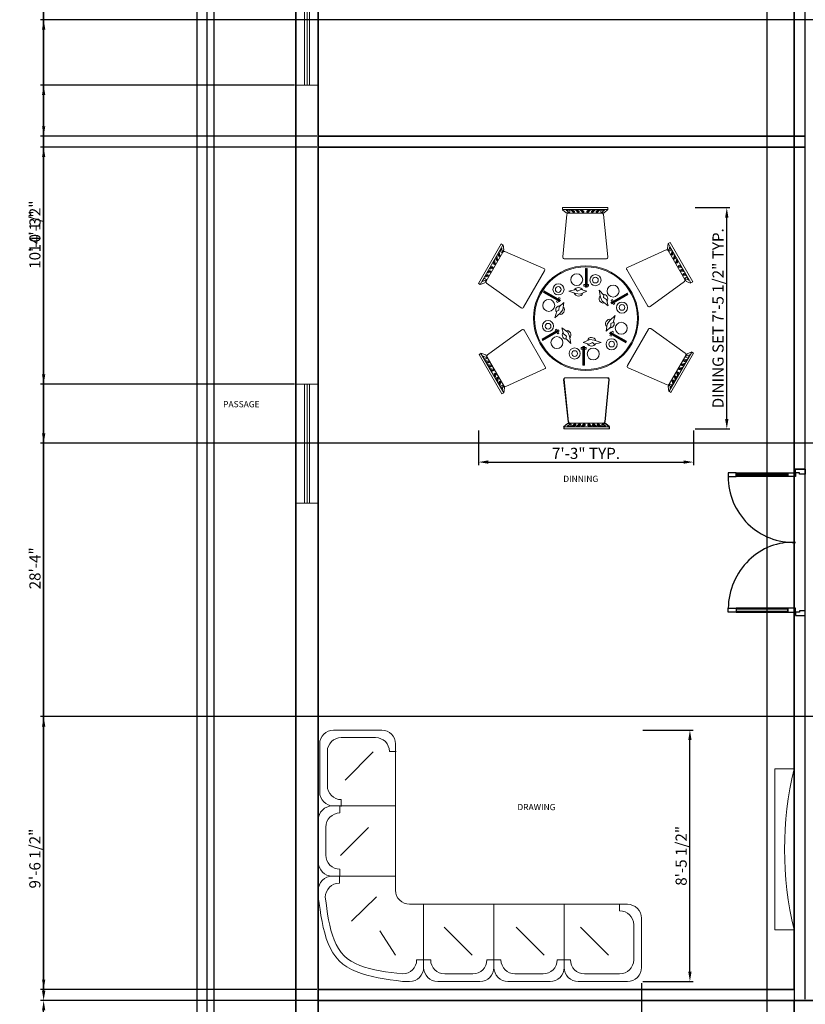
# Model space of a CAD drawing. Units: inches. Extents: x 1239 to 2276906, y 2273 to 321338.
# Tile 10 of 23: x 1239 to 1556, y 2629 to 3026. Entities that reach past the tile are written whole.
import ezdxf

# ---------------------------------------------------------------- set-up
doc = ezdxf.new("R2010")
doc.units = ezdxf.units.IN
for name, color, linetype, lineweight in [('A-ANNO-DIMS', 2, 'Continuous', 18), ('A-AREA-IDEN', 7, 'Continuous', 18), ('A-FLOR-CASE', 8, 'Continuous', 18), ('A-FLOR-PORCH', 7, 'Continuous', 25), ('A-FURN', 8, 'Continuous', 13), ('C-PROP', 7, 'Continuous', 25), ('DOOR', 1, 'Continuous', 25), ('wall', 7, 'Continuous', 35), ('WINDOW', 50, 'Continuous', 18)]:
    doc.layers.add(name, color=color, linetype=linetype, lineweight=lineweight)
doc.styles.get("Standard").update_dxf_attribs({"font": 'arial.ttf'})
doc.dimstyles.new('ISO-25', dxfattribs={"dimtxt": 4.5, "dimasz": 4, "dimexe": 1.25, "dimexo": 0.625, "dimtad": 1, "dimdec": 1, "dimlunit": 3, "dimtxsty": 'Standard', "dimcen": 2.5, "dimadec": 0, "dimazin": 0, "dimtfac": 1, "dimtdec": 1, "dimtmove": 0, "dimatfit": 3, "dimfxl": 1, "dimarcsym": 0})

# ---------------------------------------------------------------- blocks, each defined once
blk = doc.blocks.new('A$C4B324E0D')
for points in [[(-0.4032, -0.0374), (-0.3959, 0.0153), (-0.3883, 0.0678), (-0.3801, 0.1195), (-0.3709, 0.1704), (-0.3605, 0.22), (-0.3485, 0.2679), (-0.3346, 0.314), (-0.3185, 0.3579), (-0.2998, 0.3993), (-0.2783, 0.4378), (-0.2537, 0.4731), (-0.2255, 0.5049), (-0.1936, 0.5331), (-0.1583, 0.5578), (-0.1198, 0.5793), (-0.0785, 0.5979), (-0.0346, 0.614), (0.0115, 0.628), (0.0595, 0.64), (0.1091, 0.6504), (0.1599, 0.6595), (0.2117, 0.6678), (0.2641, 0.6753), (0.3168, 0.6826)], [(0.3768, 0.6826), (0.3168, 0.6826)], [(0.9768, 0.6826), (0.6168, 0.6826)], [(1.5769, 0.6826), (1.2168, 0.6826)], [(1.8168, 0.6826), (2.2368, 0.6826)], [(-0.3432, -0.0374), (-0.3369, 0.0114), (-0.3303, 0.0599), (-0.3232, 0.1078), (-0.3151, 0.1548), (-0.3059, 0.2006), (-0.2951, 0.2449), (-0.2826, 0.2874), (-0.2681, 0.3278), (-0.2511, 0.3658), (-0.2315, 0.4011), (-0.2089, 0.4335), (-0.1831, 0.4625), (-0.1538, 0.488), (-0.1214, 0.5102), (-0.086, 0.5294), (-0.0479, 0.546), (-0.0075, 0.5602), (0.035, 0.5722), (0.0793, 0.5825), (0.125, 0.5914), (0.172, 0.599), (0.2198, 0.6057), (0.2682, 0.6119), (0.3168, 0.6177)], [(0.3168, 0.6177), (0.3168, 0.6177)], [(0.9168, 0.6177), (0.6768, 0.6177)], [(1.5168, 0.6177), (1.2768, 0.6177)], [(2.1704, 0.6177), (1.8704, 0.6177)], [(0.4968, 0.0226), (0.4968, 0.5626)], [(0.4968, 0.5626), (0.4968, 0.0226), (1.0968, 0.0226)], [(1.0968, 0.5626), (1.0968, 0.0226), (1.6968, 0.0226)], [(1.0968, 0.0226), (1.0968, 0.5626)], [(1.6968, 0.0226), (1.6968, 0.5626)], [(2.2368, 0.0226), (1.6968, 0.0226), (1.6968, 0.5626)], [(2.3569, 0.5626), (2.3569, 0.1426)], [(0.255, 0.4573), (0.1211, 0.2495)], [(0.4968, 0.4977), (0.4368, 0.4977), (0.4368, 0.4977)], [(0.5569, 0.4977), (0.5569, 0.4977), (0.4968, 0.4977)], [(0.9111, 0.4573), (0.6711, 0.2173)], [(1.0968, 0.4977), (1.0368, 0.4977), (1.0368, 0.4977)], [(1.1569, 0.4977), (1.1569, 0.4977), (1.0968, 0.4977)], [(1.527, 0.4573), (1.287, 0.2173)], [(1.6969, 0.4977), (1.6368, 0.4977), (1.6368, 0.4977)], [(1.7504, 0.4977), (1.7504, 0.4977), (1.6904, 0.4977)], [(2.0759, 0.4573), (1.8359, 0.2173)], [(2.2904, 0.1977), (2.2904, 0.4977)], [(-0.1199, 0.1664), (0.0943, -0.0414)], [(0.4968, 0.0226), (0.3768, 0.0226)], [(2.1704, 0.0177), (2.1704, 0.0777), (2.1704, 0.0777)], [(-0.4032, -0.0974), (-0.4032, -0.0374)], [(-0.3432, -0.0374), (-0.3432, -0.0374)], [(-0.2232, -0.2174), (-0.2232, -0.1574), (-0.2232, -0.1574)], [(0.2568, -0.0974), (0.2568, -0.2174)], [(-0.2832, -0.8174), (0.2568, -0.8174), (0.2568, -0.2174)], [(0.2568, -0.2174), (-0.2832, -0.2174)], [(0.2568, -0.2174), (-0.2832, -0.2174)], [(-0.2183, -0.2174), (-0.2183, -0.2774), (-0.2183, -0.2774)], [(-0.4032, -0.3374), (-0.4032, -0.6974)], [(-0.3383, -0.3974), (-0.3383, -0.6374)], [(-0.2136, -0.3946), (0.0264, -0.6346)], [(0.2568, -0.8174), (-0.2832, -0.8174)], [(-0.2732, -0.8174), (0.2568, -0.8174), (0.2568, -1.3475)], [(-0.2183, -0.7574), (-0.2183, -0.7574), (-0.2183, -0.8174)], [(-0.208, -0.8126), (-0.208, -0.8715), (-0.208, -0.8715)], [(0.2568, -0.8174), (0.2568, -1.3475)], [(-0.391, -1.3475), (-0.391, -0.9352)], [(-0.3258, -0.9893), (-0.3258, -1.2838)], [(-0.1734, -1.0387), (0.0666, -1.2787)], [(0.2043, -1.2838), (0.2043, -1.2838), (0.2632, -1.2838)], [(-0.208, -1.4016), (0.0865, -1.4016)], [(0.1391, -1.4653), (-0.2732, -1.4653)]]:
    blk.add_lwpolyline(points)
for centre, radius, start, end in [((0.3768, 0.5626), 0.12, 0, 90), ((0.6168, 0.5626), 0.12, 90, 180), ((0.9768, 0.5626), 0.12, 0, 90), ((1.2168, 0.5626), 0.12, 90, 180), ((1.5769, 0.5626), 0.12, 0, 90), ((1.8168, 0.5626), 0.12, 90, 180), ((2.2368, 0.5626), 0.12, 0, 90), ((0.3168, 0.4977), 0.12, 0, 90), ((0.6768, 0.4977), 0.12, 90, 180), ((0.9168, 0.4977), 0.12, 0, 90), ((1.2768, 0.4977), 0.12, 90, 180), ((1.5168, 0.4977), 0.12, 0, 90), ((1.8704, 0.4977), 0.12, 90, 180), ((2.1704, 0.4977), 0.12, 0, 90), ((2.1704, 0.1977), 0.12, 270, 0), ((2.2368, 0.1426), 0.12, 270, 0), ((0.3768, -0.0974), 0.12, 90, 180), ((-0.2232, -0.0374), 0.12, 180, 270), ((-0.2832, -0.0974), 0.12, 179.9997, 270), ((-0.2832, -0.3374), 0.12, 90, 180), ((-0.2183, -0.3974), 0.12, 90, 180), ((-0.2183, -0.6374), 0.12, 180, 270), ((-0.2832, -0.6974), 0.12, 179.9997, 270), ((-0.2732, -0.9352), 0.1178, 90, 180), ((-0.208, -0.9893), 0.1178, 90, 180), ((-0.208, -1.2838), 0.1178, 180, 270), ((0.0865, -1.2838), 0.1178, 270, 0), ((-0.2732, -1.3475), 0.1178, 179.9997, 270), ((0.1391, -1.3475), 0.1178, 270, 0)]:
    blk.add_arc(centre, radius, start, end)
blk = doc.blocks.new('A$C58C6152E')
at = {"xscale": 1.5, "yscale": 1.5, "zscale": 1.5, "rotation": 90}
blk.add_blockref('A$C4B324E0D', (1.024, 0.605), dxfattribs=at)
blk = doc.blocks.new('A$C15DC316E')
at = {"xscale": -1, "rotation": 270}
blk.add_blockref('A$C58C6152E', (0, 0), dxfattribs=at)
blk = doc.blocks.new('A$C45501D90')
for p, q in [((-242, 1134), (224, 1134)), ((-242, 1113), (-242, 1134)), ((224, 1113), (-242, 1113)), ((-242, 1111), (-202, 1079)), ((224, 1113), (187, 1079)), ((224, 1134), (224, 1113)), ((-197, 1062), (-239, 628)), ((-204, 1106), (-166, 1108)), ((-169, 1081), (-204, 1106)), ((-202, 1079), (-169, 1081)), ((162, 1076), (-181, 1076)), ((-166, 1108), (-167, 1086)), ((-156, 1110), (-132, 1086)), ((-119, 1086), (-143, 1108)), ((-143, 1108), (-134, 1108)), ((-134, 1108), (-122, 1098)), ((-132, 1086), (-119, 1086)), ((-122, 1098), (-119, 1102)), ((-119, 1102), (-118, 1087)), ((-108, 1110), (-84, 1086)), ((-71, 1086), (-95, 1108)), ((-95, 1108), (-86, 1108)), ((-86, 1108), (-75, 1098)), ((-84, 1086), (-71, 1086)), ((-75, 1098), (-71, 1102)), ((-71, 1102), (-70, 1087)), ((-60, 1110), (-36, 1086)), ((-23, 1086), (-47, 1108)), ((-47, 1108), (-38, 1108)), ((-38, 1108), (-27, 1098)), ((-36, 1086), (-23, 1086)), ((-27, 1098), (-23, 1102)), ((-23, 1102), (-22, 1087)), ((8, 1102), (7, 1087)), ((8, 1086), (32, 1108)), ((12, 1098), (8, 1102)), ((21, 1086), (8, 1086)), ((23, 1108), (12, 1098)), ((45, 1110), (21, 1086)), ((32, 1108), (23, 1108)), ((56, 1102), (55, 1087)), ((56, 1086), (80, 1108)), ((60, 1098), (56, 1102)), ((69, 1086), (56, 1086)), ((71, 1108), (60, 1098)), ((93, 1110), (69, 1086)), ((80, 1108), (71, 1108)), ((104, 1102), (103, 1087)), ((104, 1086), (128, 1108)), ((107, 1098), (104, 1102)), ((117, 1086), (104, 1086)), ((119, 1108), (107, 1098)), ((141, 1110), (117, 1086)), ((128, 1108), (119, 1108)), ((189, 1106), (151, 1108)), ((151, 1108), (152, 1086)), ((154, 1081), (189, 1106)), ((187, 1079), (154, 1081)), ((225, 628), (178, 1062)), ((-1103, 357), (-870, 761)), ((-852, 750), (-1085, 347)), ((-864, 717), (-884, 684)), ((-870, 761), (-852, 750)), ((-859, 674), (-864, 717)), ((-849, 752), (-841, 702)), ((841, 765), (834, 715)), ((834, 715), (852, 687)), ((843, 766), (861, 776)), ((1076, 362), (843, 766)), ((852, 687), (856, 730)), ((856, 730), (877, 697)), ((861, 776), (1094, 373)), ((-851, 678), (-1023, 381)), ((-919, 624), (-924, 615)), ((-924, 615), (-921, 601)), ((-912, 592), (-919, 624)), ((-914, 635), (-906, 603)), ((-898, 642), (-902, 641)), ((-902, 641), (-890, 633)), ((-895, 665), (-900, 657)), ((-900, 657), (-898, 642)), ((-888, 633), (-895, 665)), ((-890, 677), (-882, 644)), ((-882, 644), (-888, 633)), ((-884, 684), (-864, 675)), ((-841, 702), (-859, 674)), ((-431, 509), (-831, 685)), ((-223, 610), (209, 610)), ((821, 702), (424, 521)), ((1013, 398), (841, 695)), ((877, 697), (857, 688)), ((883, 690), (874, 657)), ((874, 657), (881, 646)), ((881, 646), (888, 678)), ((894, 654), (883, 646)), ((888, 678), (893, 670)), ((893, 670), (890, 655)), ((890, 655), (894, 654)), ((907, 648), (898, 616)), ((898, 616), (904, 605)), ((904, 605), (912, 637)), ((918, 613), (907, 604)), ((912, 637), (917, 628)), ((917, 628), (914, 614)), ((914, 614), (918, 613)), ((931, 607), (922, 574)), ((-991, 503), (-958, 511)), ((-952, 522), (-983, 513)), ((-983, 513), (-978, 521)), ((-978, 521), (-965, 526)), ((-965, 526), (-966, 530)), ((-966, 530), (-953, 525)), ((-958, 511), (-952, 522)), ((-945, 559), (-950, 558)), ((-950, 558), (-938, 550)), ((-943, 582), (-948, 574)), ((-948, 574), (-945, 559)), ((-936, 550), (-943, 582)), ((-938, 594), (-930, 561)), ((-930, 561), (-936, 550)), ((-921, 601), (-926, 600)), ((-926, 600), (-914, 591)), ((-906, 603), (-912, 592)), ((-6, 509, 91), (0, 509, 91)), ((-6, 318, 91), (-6, 509, 91)), ((0, 509, 91), (0, 318, 91)), ((6, 318, 91), (6, 509, 91)), ((6, 509, 91), (12, 509, 91)), ((12, 509, 91), (12, 318, 91)), ((922, 574), (928, 563)), ((928, 563), (936, 595)), ((942, 571), (931, 563)), ((936, 595), (941, 587)), ((941, 587), (938, 572)), ((938, 572), (942, 571)), ((951, 524), (944, 535)), ((944, 535), (976, 526)), ((958, 543), (945, 538)), ((983, 516), (951, 524)), ((957, 539), (958, 543)), ((971, 534), (957, 539)), ((976, 526), (971, 534)), ((-1060, 377), (-1042, 411)), ((-1042, 411), (-1024, 398)), ((-1039, 420), (-1006, 428)), ((-1000, 440), (-1031, 430)), ((-1031, 430), (-1026, 438)), ((-1026, 438), (-1012, 443)), ((-1015, 461), (-982, 470)), ((-1012, 443), (-1014, 448)), ((-1014, 448), (-1000, 442)), ((-976, 481), (-1007, 471)), ((-1007, 471), (-1002, 480)), ((-1006, 428), (-1000, 440)), ((-1002, 480), (-989, 485)), ((-989, 485), (-990, 489)), ((-990, 489), (-976, 483)), ((-982, 470), (-976, 481)), ((-640, 112), (-424, 486)), ((417, 498), (633, 124)), ((968, 494), (1000, 484)), ((975, 483), (968, 494)), ((982, 502), (969, 496)), ((1007, 474), (975, 483)), ((981, 498), (982, 502)), ((995, 493), (981, 498)), ((999, 441), (992, 453)), ((992, 453), (1024, 443)), ((1006, 461), (993, 455)), ((1000, 484), (995, 493)), ((1031, 433), (999, 441)), ((1005, 456), (1006, 461)), ((1019, 451), (1005, 456)), ((1028, 377), (1013, 407)), ((1013, 407), (1053, 390)), ((1035, 424), (1016, 411)), ((1024, 443), (1019, 451)), ((1053, 390), (1035, 424)), ((-1085, 347), (-1103, 357)), ((-1083, 346), (-1036, 364)), ((-1020, 394), (-1060, 377)), ((-1036, 364), (-1020, 394)), ((-1018, 360), (-663, 107)), ((-22, 329, 91), (-22, 345, 91)), ((-22, 345, 91), (-6, 345, 91)), ((-6, 329, 91), (-22, 329, 91)), ((0, 318, 91), (-6, 318, 91)), ((0, 345, 91), (6, 345, 91)), ((6, 329, 91), (0, 329, 91)), ((12, 318, 91), (6, 318, 91)), ((12, 345, 91), (27, 345, 91)), ((27, 329, 91), (12, 329, 91)), ((27, 345, 91), (27, 329, 91)), ((656, 119), (1008, 377)), ((1076, 359), (1028, 377)), ((1094, 373), (1076, 362)), ((-436, 265, 91), (-433, 271, 91)), ((-271, 170, 91), (-436, 265, 91)), ((-433, 271, 91), (-268, 175, 91)), ((-431, 275, 91), (-428, 280, 91)), ((-265, 180, 91), (-431, 275, 91)), ((-428, 280, 91), (-262, 185, 91)), ((-286, 198, 91), (-278, 212, 91)), ((-278, 212, 91), (-264, 204, 91)), ((-264, 204, 91), (-272, 191, 91)), ((-175, 276, 91), (-105, 293, 91)), ((-103, 252, 91), (-175, 276, 91)), ((-105, 293, 91), (-86, 278, 91)), ((-60, 246, 91), (-103, 252, 91)), ((-86, 278, 91), (-52, 294, 91)), ((9, 276, 91), (-60, 246, 91)), ((-52, 294, 91), (9, 276, 91)), ((134, 288, 91), (184, 236, 91)), ((150, 214, 91), (134, 288, 91)), ((166, 173, 91), (150, 214, 91)), ((184, 236, 91), (181, 211, 91)), ((181, 211, 91), (211, 190, 91)), ((255, 162, 91), (421, 257, 91)), ((424, 252, 91), (258, 157, 91)), ((261, 152, 91), (426, 248, 91)), ((429, 242, 91), (264, 147, 91)), ((421, 257, 91), (424, 252, 91)), ((426, 248, 91), (429, 242, 91)), ((-303, 169, 91), (-294, 183, 91)), ((-289, 161, 91), (-303, 169, 91)), ((-291, 188, 91), (-289, 193, 91)), ((-281, 176, 91), (-289, 161, 91)), ((-275, 185, 91), (-278, 181, 91)), ((-277, 81, 91), (-274, 118, 91)), ((-274, 118, 91), (-227, 162, 91)), ((-268, 175, 91), (-271, 170, 91)), ((-262, 185, 91), (-265, 180, 91)), ((-227, 162, 91), (-236, 87, 91)), ((227, 128, 91), (166, 173, 91)), ((211, 190, 91), (227, 128, 91)), ((258, 157, 91), (255, 162, 91)), ((257, 182, 91), (270, 190, 91)), ((265, 168, 91), (257, 182, 91)), ((264, 147, 91), (261, 152, 91)), ((271, 158, 91), (268, 162, 91)), ((270, 190, 91), (278, 175, 91)), ((281, 139, 91), (274, 153, 91)), ((281, 170, 91), (284, 165, 91)), ((295, 147, 91), (281, 139, 91)), ((287, 160, 91), (295, 147, 91)), ((-320, 2, 91), (-299, 72, 91)), ((-263, 53, 91), (-320, 2, 91)), ((-299, 72, 91), (-277, 81, 91)), ((-236, 87, 91), (-263, 53, 91)), ((243, -25, 91), (299, 26, 91)), ((299, 26, 91), (279, -44, 91)), ((-247, -100, 91), (-187, -145, 91)), ((-232, -162, 91), (-247, -100, 91)), ((207, -134, 91), (216, -60, 91)), ((253, -90, 91), (207, -134, 91)), ((216, -60, 91), (243, -25, 91)), ((256, -53, 91), (253, -90, 91)), ((279, -44, 91), (256, -53, 91)), ((-656, -119), (-1008, -377)), ((-417, -498), (-633, -124)), ((-450, -214, 91), (-284, -119, 91)), ((-281, -124, 91), (-447, -220, 91)), ((-444, -224, 91), (-279, -129, 91)), ((-276, -134, 91), (-441, -229, 91)), ((-315, -119, 91), (-302, -111, 91)), ((-307, -132, 91), (-315, -119, 91)), ((-302, -142, 91), (-304, -137, 91)), ((-302, -111, 91), (-294, -125, 91)), ((-290, -162, 91), (-299, -147, 91)), ((-291, -130, 91), (-288, -134, 91)), ((-277, -154, 91), (-290, -162, 91)), ((-285, -140, 91), (-277, -154, 91)), ((-284, -119, 91), (-281, -124, 91)), ((-279, -129, 91), (-276, -134, 91)), ((-201, -183, 91), (-232, -162, 91)), ((-205, -208, 91), (-201, -183, 91)), ((-187, -145, 91), (-170, -186, 91)), ((-170, -186, 91), (-155, -260, 91)), ((242, -157, 91), (245, -152, 91)), ((407, -252, 91), (242, -157, 91)), ((244, -176, 91), (252, -163, 91)), ((257, -184, 91), (244, -176, 91)), ((245, -152, 91), (410, -247, 91)), ((248, -147, 91), (251, -142, 91)), ((413, -243, 91), (248, -147, 91)), ((251, -142, 91), (416, -237, 91)), ((255, -157, 91), (257, -153, 91)), ((265, -170, 91), (257, -184, 91)), ((260, -148, 91), (269, -133, 91)), ((271, -160, 91), (268, -165, 91)), ((269, -133, 91), (282, -141, 91)), ((282, -141, 91), (274, -155, 91)), ((640, -112), (424, -486)), ((1018, -360), (663, -107)), ((-447, -220, 91), (-450, -214, 91)), ((-441, -229, 91), (-444, -224, 91)), ((-155, -260, 91), (-205, -208, 91)), ((-48, -317, 91), (-48, -301, 91)), ((-48, -301, 91), (-32, -301, 91)), ((-32, -481, 91), (-32, -290, 91)), ((-32, -290, 91), (-26, -290, 91)), ((-30, -248, 91), (39, -218, 91)), ((32, -266, 91), (-30, -248, 91)), ((-26, -290, 91), (-26, -481, 91)), ((-26, -301, 91), (-21, -301, 91)), ((-21, -481, 91), (-21, -290, 91)), ((-21, -290, 91), (-15, -290, 91)), ((-15, -290, 91), (-15, -481, 91)), ((-15, -301, 91), (2, -301, 91)), ((2, -301, 91), (2, -317, 91)), ((65, -250, 91), (32, -266, 91)), ((39, -218, 91), (83, -224, 91)), ((84, -265, 91), (65, -250, 91)), ((83, -224, 91), (155, -248, 91)), ((155, -248, 91), (84, -265, 91)), ((410, -247, 91), (407, -252, 91)), ((416, -237, 91), (413, -243, 91)), ((-1094, -373), (-1076, -362)), ((-861, -776), (-1094, -373)), ((-1076, -359), (-1028, -377)), ((-1076, -362), (-843, -766)), ((-1053, -390), (-1035, -424)), ((-1013, -407), (-1053, -390)), ((-1028, -377), (-1013, -407)), ((-1013, -398), (-841, -695)), ((-32, -317, 91), (-48, -317, 91)), ((-21, -317, 91), (-26, -317, 91)), ((2, -317, 91), (-15, -317, 91)), ((851, -678), (1023, -381)), ((852, -750), (1085, -347)), ((1103, -357), (870, -761)), ((1036, -364), (1020, -394)), ((1020, -394), (1060, -377)), ((1042, -411), (1024, -398)), ((1083, -346), (1036, -364)), ((1060, -377), (1042, -411)), ((1085, -347), (1103, -357)), ((-1035, -424), (-1016, -411)), ((-1031, -433), (-999, -441)), ((-1024, -443), (-1019, -451)), ((-992, -453), (-1024, -443)), ((-1019, -451), (-1005, -456)), ((-1007, -474), (-975, -483)), ((-1006, -461), (-993, -455)), ((-1005, -456), (-1006, -461)), ((-968, -494), (-1000, -484)), ((-1000, -484), (-995, -493)), ((-999, -441), (-992, -453)), ((-995, -493), (-981, -498)), ((-982, -502), (-969, -496)), ((-981, -498), (-982, -502)), ((-975, -483), (-968, -494)), ((-26, -481, 91), (-32, -481, 91)), ((-15, -481, 91), (-21, -481, 91)), ((991, -503), (958, -511)), ((982, -470), (976, -481)), ((976, -481), (1007, -471)), ((990, -489), (976, -483)), ((1015, -461), (982, -470)), ((1002, -480), (989, -485)), ((989, -485), (990, -489)), ((1006, -428), (1000, -440)), ((1000, -440), (1031, -430)), ((1014, -448), (1000, -442)), ((1007, -471), (1002, -480)), ((1039, -420), (1006, -428)), ((1026, -438), (1012, -443)), ((1012, -443), (1014, -448)), ((1031, -430), (1026, -438)), ((-983, -516), (-951, -524)), ((-944, -535), (-976, -526)), ((-976, -526), (-971, -534)), ((-971, -534), (-957, -539)), ((-958, -543), (-945, -538)), ((-957, -539), (-958, -543)), ((-951, -524), (-944, -535)), ((-942, -571), (-931, -563)), ((-938, -572), (-942, -571)), ((-941, -587), (-938, -572)), ((-936, -595), (-941, -587)), ((-928, -563), (-936, -595)), ((-931, -607), (-922, -574)), ((-922, -574), (-928, -563)), ((-918, -613), (-907, -604)), ((-904, -605), (-912, -637)), ((-898, -616), (-904, -605)), ((-821, -702), (-424, -521)), ((431, -509), (831, -685)), ((906, -603), (912, -592)), ((914, -635), (906, -603)), ((912, -592), (919, -624)), ((926, -600), (914, -591)), ((921, -601), (926, -600)), ((924, -615), (921, -601)), ((930, -561), (936, -550)), ((938, -594), (930, -561)), ((936, -550), (943, -582)), ((950, -558), (938, -550)), ((943, -582), (948, -574)), ((945, -559), (950, -558)), ((948, -574), (945, -559)), ((958, -511), (952, -522)), ((952, -522), (983, -513)), ((966, -530), (953, -525)), ((978, -521), (965, -526)), ((965, -526), (966, -530)), ((983, -513), (978, -521)), ((-914, -614), (-918, -613)), ((-917, -628), (-914, -614)), ((-912, -637), (-917, -628)), ((-907, -648), (-898, -616)), ((-894, -654), (-883, -646)), ((-890, -655), (-894, -654)), ((-893, -670), (-890, -655)), ((-888, -678), (-893, -670)), ((-881, -646), (-888, -678)), ((-883, -690), (-874, -657)), ((-874, -657), (-881, -646)), ((-877, -697), (-857, -688)), ((-856, -730), (-877, -697)), ((-852, -687), (-856, -730)), ((-834, -715), (-852, -687)), ((-229, -629), (-182, -1063)), ((-225, -628), (-178, -1062)), ((219, -612), (-213, -612)), ((223, -610), (-209, -610)), ((193, -1063), (235, -629)), ((197, -1062), (239, -628)), ((841, -702), (859, -674)), ((849, -752), (841, -702)), ((859, -674), (864, -717)), ((884, -684), (864, -675)), ((864, -717), (884, -684)), ((882, -644), (888, -633)), ((890, -677), (882, -644)), ((888, -633), (895, -665)), ((902, -641), (890, -633)), ((895, -665), (900, -657)), ((898, -642), (902, -641)), ((900, -657), (898, -642)), ((919, -624), (924, -615)), ((-843, -766), (-861, -776)), ((-841, -765), (-834, -715)), ((870, -761), (852, -750)), ((-231, -1113), (-191, -1081)), ((-227, -1111), (-187, -1079)), ((-158, -1082), (-193, -1108)), ((-193, -1108), (-155, -1109)), ((-191, -1081), (-158, -1082)), ((-154, -1081), (-189, -1106)), ((-189, -1106), (-151, -1108)), ((-187, -1079), (-154, -1081)), ((-166, -1078), (177, -1078)), ((-162, -1076), (181, -1076)), ((-155, -1109), (-156, -1087)), ((-151, -1108), (-152, -1086)), ((-145, -1111), (-121, -1087)), ((-141, -1110), (-117, -1086)), ((-108, -1087), (-132, -1109)), ((-132, -1109), (-123, -1109)), ((-104, -1086), (-128, -1108)), ((-128, -1108), (-119, -1108)), ((-123, -1109), (-112, -1100)), ((-121, -1087), (-108, -1087)), ((-119, -1108), (-107, -1098)), ((-117, -1086), (-104, -1086)), ((-112, -1100), (-108, -1103)), ((-108, -1103), (-107, -1089)), ((-107, -1098), (-104, -1102)), ((-104, -1102), (-103, -1087)), ((-97, -1111), (-73, -1087)), ((-93, -1110), (-69, -1086)), ((-60, -1087), (-84, -1109)), ((-84, -1109), (-75, -1109)), ((-56, -1086), (-80, -1108)), ((-80, -1108), (-71, -1108)), ((-75, -1109), (-64, -1100)), ((-73, -1087), (-60, -1087)), ((-71, -1108), (-60, -1098)), ((-69, -1086), (-56, -1086)), ((-64, -1100), (-60, -1103)), ((-60, -1103), (-59, -1089)), ((-60, -1098), (-56, -1102)), ((-56, -1102), (-55, -1087)), ((-49, -1111), (-25, -1087)), ((-45, -1110), (-21, -1086)), ((-13, -1087), (-37, -1109)), ((-37, -1109), (-27, -1109)), ((-8, -1086), (-32, -1108)), ((-32, -1108), (-23, -1108)), ((-27, -1109), (-16, -1100)), ((-25, -1087), (-13, -1087)), ((-23, -1108), (-12, -1098)), ((-21, -1086), (-8, -1086)), ((-16, -1100), (-13, -1103)), ((-13, -1103), (-11, -1089)), ((-12, -1098), (-8, -1102)), ((-8, -1102), (-7, -1087)), ((19, -1103), (18, -1089)), ((19, -1087), (43, -1109)), ((32, -1087), (19, -1087)), ((23, -1100), (19, -1103)), ((23, -1102), (22, -1087)), ((23, -1086), (47, -1108)), ((36, -1086), (23, -1086)), ((27, -1098), (23, -1102)), ((34, -1109), (23, -1100)), ((38, -1108), (27, -1098)), ((56, -1111), (32, -1087)), ((43, -1109), (34, -1109)), ((60, -1110), (36, -1086)), ((47, -1108), (38, -1108)), ((67, -1103), (66, -1089)), ((67, -1087), (91, -1109)), ((80, -1087), (67, -1087)), ((70, -1100), (67, -1103)), ((71, -1102), (70, -1087)), ((82, -1109), (70, -1100)), ((71, -1086), (95, -1108)), ((84, -1086), (71, -1086)), ((75, -1098), (71, -1102)), ((86, -1108), (75, -1098)), ((104, -1111), (80, -1087)), ((91, -1109), (82, -1109)), ((108, -1110), (84, -1086)), ((95, -1108), (86, -1108)), ((115, -1103), (114, -1089)), ((115, -1087), (139, -1109)), ((128, -1087), (115, -1087)), ((118, -1100), (115, -1103)), ((119, -1102), (118, -1087)), ((130, -1109), (118, -1100)), ((119, -1086), (143, -1108)), ((132, -1086), (119, -1086)), ((122, -1098), (119, -1102)), ((134, -1108), (122, -1098)), ((152, -1111), (128, -1087)), ((139, -1109), (130, -1109)), ((156, -1110), (132, -1086)), ((143, -1108), (134, -1108)), ((161, -1109), (163, -1087)), ((200, -1108), (161, -1109)), ((198, -1081), (165, -1082)), ((165, -1082), (200, -1108)), ((166, -1108), (167, -1086)), ((204, -1106), (166, -1108)), ((202, -1079), (169, -1081)), ((169, -1081), (204, -1106)), ((238, -1113), (198, -1081)), ((242, -1111), (202, -1079)), ((-228, -1114), (238, -1114)), ((-228, -1135), (-228, -1114)), ((238, -1135), (-228, -1135)), ((-224, -1113), (242, -1113)), ((-224, -1134), (-224, -1113)), ((242, -1134), (-224, -1134)), ((238, -1114), (238, -1135)), ((242, -1113), (242, -1134))]:
    blk.add_line(p, q)
for centre, radius in [((0, 0), 537), ((0, 0), 527), ((-95, 395, 91), 61.3), ((97, 390, 91), 56.9), ((96, 391, 91), 29.4), ((-282, 295, 91), 56.9), ((-284, 294, 91), 29.4), ((277, 278, 91), 61.3), ((-382, 131, 91), 61.3), ((369, 109, 91), 56.9), ((369, 111, 91), 29.4), ((-389, -81, 91), 56.9), ((-389, -83, 91), 29.4), ((362, -103, 91), 61.3), ((-298, -250, 91), 61.3), ((262, -267, 91), 56.9), ((263, -266, 91), 29.4), ((-117, -362, 91), 56.9), ((-116, -363, 91), 29.4), ((74, -367, 91), 61.3)]:
    blk.add_circle(centre, radius)
for centre, radius, start, end in [((-181, 1060), 16, 90, 174.5199), ((162, 1060), 16, 6.2572, 90), ((-837, 670), 16, 66.2572, 150), ((-223, 626), 16, 174.5199, 270), ((209, 626), 16, 270, 6.2572), ((827, 687), 16, 30, 114.5199), ((-438, 494), 16, 330, 66.2572), ((431, 506), 16, 114.5199, 210), ((-1009, 373), 16, 150, 234.5199), ((-77, 270, 91), 44.6, 25.8558, 153.3359), ((999, 390), 16, 306.2572, 30), ((-77, 270, 91), 44.6, 195.9338, 342.9389), ((178, 200, 91), 44.6, 135.9338, 282.9389), ((178, 200, 91), 44.6, 325.8558, 93.3359), ((-654, 120), 16, 234.5199, 330), ((-266, 84, 91), 44.6, 85.8558, 213.3359), ((-266, 84, 91), 44.6, 255.9338, 42.9389), ((647, 132), 16, 210, 306.2572), ((245, -56, 91), 44.6, 75.9338, 222.9389), ((245, -56, 91), 44.6, 265.8558, 33.3359), ((-647, -132), 16, 30, 126.2572), ((-198, -172, 91), 44.6, 145.8558, 273.3359), ((-198, -172, 91), 44.6, 315.9338, 102.9389), ((57, -242, 91), 44.6, 15.9338, 162.9389), ((654, -120), 16, 54.5199, 150), ((57, -242, 91), 44.6, 205.8558, 333.3359), ((-999, -390), 16, 126.2572, 210), ((1009, -373), 16, 330, 54.5199), ((-431, -506), 16, 294.5199, 30), ((438, -494), 16, 150, 246.2572), ((-827, -687), 16, 210, 294.5199), ((-213, -628), 16, 90, 186.2572), ((-209, -626), 16, 90, 186.2572), ((219, -628), 16, 354.5199, 90), ((223, -626), 16, 354.5199, 90), ((837, -670), 16, 246.2572, 330), ((-166, -1062), 16, 186.2572, 270), ((-162, -1060), 16, 186.2572, 270), ((177, -1062), 16, 270, 354.5199), ((181, -1060), 16, 270, 354.5199)]:
    blk.add_arc(centre, radius, start, end)
blk = doc.blocks.new('DOOR-DOUBLE-60')
for p, q in [((1.38, 27.95), (1.38, 31.1)), ((1.38, 31.1), (2.95, 31.1)), ((1.38, 27.95), (1.38, 7.09)), ((2.95, 27.95), (1.38, 27.95)), ((2.95, 27.95), (1.38, 27.95)), ((1.77, 27.95), (1.77, 7.09)), ((2.56, 27.95), (1.77, 27.95)), ((2.56, 7.09), (2.56, 27.95)), ((2.95, 31.1), (2.95, 27.95)), ((2.95, 7.09), (2.95, 27.95)), ((56.1, 31.1), (56.1, 27.95)), ((57.68, 31.1), (56.1, 31.1)), ((56.1, 27.95), (57.68, 27.95)), ((56.1, 7.09), (56.1, 27.95)), ((56.1, 27.95), (57.68, 27.95)), ((56.5, 7.09), (56.5, 27.95)), ((56.5, 27.95), (57.28, 27.95)), ((57.28, 27.95), (57.28, 7.09)), ((57.68, 27.95), (57.68, 31.1)), ((57.68, 27.95), (57.68, 7.09)), ((1.38, 7.09), (1.38, 3.94)), ((2.95, 7.09), (1.38, 7.09)), ((1.38, 7.09), (2.95, 7.09)), ((1.77, 7.09), (2.56, 7.09)), ((2.95, 3.94), (2.95, 7.09)), ((57.68, 7.09), (56.1, 7.09)), ((56.1, 3.94), (56.1, 7.09)), ((56.1, 7.09), (57.68, 7.09)), ((57.28, 7.09), (56.5, 7.09)), ((57.68, 7.09), (57.68, 3.94)), ((0, 3.94), (0, 0)), ((1.38, 3.94), (0, 3.94)), ((0, 0), (1.97, 0)), ((1.38, 3.94), (2.95, 3.94)), ((1.38, 2.36), (1.38, 3.94)), ((1.97, 2.36), (1.38, 2.36)), ((1.97, 1.97), (1.97, 2.36)), ((1.97, 0), (1.97, 1.97)), ((57.68, 3.94), (56.1, 3.94)), ((57.09, 1.97), (57.09, 2.36)), ((57.09, 2.36), (57.68, 2.36)), ((57.09, 0), (57.09, 1.97)), ((59.06, 0), (57.09, 0)), ((57.68, 3.94), (59.06, 3.94)), ((57.68, 2.36), (57.68, 3.94)), ((59.06, 3.94), (59.06, 0))]:
    blk.add_line(p, q)
blk.add_arc((55.99, 4.6), 26.5, 89.7657, 181.4438)
blk.add_ellipse((2.91, 5.95), major_axis=(26.26, -4.79), ratio=0.940794, start_param=0.11153, end_param=1.73917)
blk = doc.blocks.new('WIN-48')
for p, q in [((0, 48), (9, 48)), ((0, 0), (0, 48)), ((3.5, 0), (3.5, 48)), ((4.5, 0), (4.5, 48)), ((5.5, 0), (5.5, 48)), ((9, 0), (9, 48)), ((0, 0), (9, 0))]:
    blk.add_line(p, q)
blk = doc.blocks.new('*D60')
at = {"layer": 'A-ANNO-DIMS', "color": 0, "lineweight": -2, "transparency": 16777216}
for p, q in [((1511.44, 2950.51), (1525.46, 2950.51)), ((1524.21, 2865.2), (1524.21, 2946.51)), ((1511.44, 2861.2), (1525.46, 2861.2))]:
    blk.add_line(p, q, dxfattribs=at)
at = {"layer": 'A-ANNO-DIMS', "color": 0, "transparency": 16777216}
for points in [[(1523.54, 2946.51), (1524.88, 2946.51), (1524.21, 2950.51)], [(1523.54, 2865.2), (1524.88, 2865.2), (1524.21, 2861.2)]]:
    blk.add_solid(points, dxfattribs=at)
at = {"layer": 'Defpoints', "color": 0, "transparency": 16777216}
for p in [(1510.81, 2950.51), (1524.21, 2950.51), (1510.81, 2861.2)]:
    blk.add_point(p, dxfattribs=at)
at = {"layer": 'A-ANNO-DIMS', "color": 0, "transparency": 16777216, "insert": (1521.26, 2905.86), "char_height": 4.5, "attachment_point": 5, "rotation": 90}
blk.add_mtext('DINING SET 7\'-5 1/2" TYP.', dxfattribs=at)
blk = doc.blocks.new('*D61')
at = {"layer": 'A-ANNO-DIMS', "color": 0, "lineweight": -2, "transparency": 16777216}
for p, q in [((1423.98, 2860.58), (1423.98, 2846.55)), ((1510.81, 2860.58), (1510.81, 2846.55)), ((1427.98, 2847.8), (1506.81, 2847.8))]:
    blk.add_line(p, q, dxfattribs=at)
at = {"layer": 'A-ANNO-DIMS', "color": 0, "transparency": 16777216}
for points in [[(1427.98, 2848.47), (1427.98, 2847.14), (1423.98, 2847.8)], [(1506.81, 2848.47), (1506.81, 2847.14), (1510.81, 2847.8)]]:
    blk.add_solid(points, dxfattribs=at)
at = {"layer": 'Defpoints', "color": 0, "transparency": 16777216}
for p in [(1423.98, 2861.2), (1510.81, 2861.2), (1510.81, 2847.8)]:
    blk.add_point(p, dxfattribs=at)
at = {"layer": 'A-ANNO-DIMS', "color": 0, "transparency": 16777216, "insert": (1467.4, 2850.73), "char_height": 4.5, "attachment_point": 5}
blk.add_mtext('7\'-3" TYP.', dxfattribs=at)
blk = doc.blocks.new('*D62')
at = {"layer": 'A-ANNO-DIMS', "color": 0, "lineweight": -2, "transparency": 16777216}
for p, q in [((1359.38, 2637.47), (1359.38, 2617.29)), ((1489.78, 2637.47), (1489.78, 2617.29)), ((1363.38, 2618.54), (1485.78, 2618.54))]:
    blk.add_line(p, q, dxfattribs=at)
at = {"layer": 'A-ANNO-DIMS', "color": 0, "transparency": 16777216}
for points in [[(1363.38, 2619.2), (1363.38, 2617.87), (1359.38, 2618.54)], [(1485.78, 2619.2), (1485.78, 2617.87), (1489.78, 2618.54)]]:
    blk.add_solid(points, dxfattribs=at)
at = {"layer": 'Defpoints', "color": 0, "transparency": 16777216}
for p in [(1359.38, 2638.1), (1489.78, 2638.1), (1489.78, 2618.54)]:
    blk.add_point(p, dxfattribs=at)
at = {"layer": 'A-ANNO-DIMS', "color": 0, "transparency": 16777216, "insert": (1424.58, 2621.49), "char_height": 4.5, "attachment_point": 5}
blk.add_mtext('CORNER SOFA 10\'-10 1/2"', dxfattribs=at)
blk = doc.blocks.new('*D63')
at = {"layer": 'A-ANNO-DIMS', "color": 0, "lineweight": -2, "transparency": 16777216}
for p, q in [((1490.4, 2739.57), (1510.59, 2739.57)), ((1509.34, 2642.1), (1509.34, 2735.57)), ((1490.4, 2638.1), (1510.59, 2638.1))]:
    blk.add_line(p, q, dxfattribs=at)
at = {"layer": 'A-ANNO-DIMS', "color": 0, "transparency": 16777216}
for points in [[(1508.67, 2735.57), (1510, 2735.57), (1509.34, 2739.57)], [(1508.67, 2642.1), (1510, 2642.1), (1509.34, 2638.1)]]:
    blk.add_solid(points, dxfattribs=at)
at = {"layer": 'Defpoints', "color": 0, "transparency": 16777216}
for p in [(1489.78, 2739.57), (1509.34, 2739.57), (1489.78, 2638.1)]:
    blk.add_point(p, dxfattribs=at)
at = {"layer": 'A-ANNO-DIMS', "color": 0, "transparency": 16777216, "insert": (1506.38, 2688.83), "char_height": 4.5, "attachment_point": 5, "rotation": 90}
blk.add_mtext('8\'-5 1/2"', dxfattribs=at)
blk = doc.blocks.new('*D82')
at = {"layer": 'A-ANNO-DIMS', "color": 0, "lineweight": -2, "transparency": 16777216}
for p, q in [((1349.76, 3505.9), (1247.33, 3505.9)), ((1248.58, 3501.9), (1248.58, 2634.4)), ((1358.76, 2630.4), (1247.33, 2630.4))]:
    blk.add_line(p, q, dxfattribs=at)
at = {"layer": 'A-ANNO-DIMS', "color": 0, "transparency": 16777216}
for points in [[(1247.92, 3501.9), (1249.25, 3501.9), (1248.58, 3505.9)], [(1247.92, 2634.4), (1249.25, 2634.4), (1248.58, 2630.4)]]:
    blk.add_solid(points, dxfattribs=at)
at = {"layer": 'Defpoints', "color": 0, "transparency": 16777216}
for p in [(1350.38, 3505.9), (1248.58, 2630.4), (1359.38, 2630.4)]:
    blk.add_point(p, dxfattribs=at)
at = {"layer": 'A-ANNO-DIMS', "color": 0, "transparency": 16777216, "insert": (1245.63, 3068.15), "char_height": 4.5, "attachment_point": 5, "rotation": 90}
blk.add_mtext('72\'-11 1/2"', dxfattribs=at)
blk = doc.blocks.new('*D89')
at = {"layer": 'A-ANNO-DIMS', "color": 0, "lineweight": -2, "transparency": 16777216}
for p, q in [((1359.38, 3215.77), (1359.38, 2275.7)), ((1551.38, 3215.77), (1551.38, 2275.7)), ((1363.38, 2276.95), (1547.38, 2276.95))]:
    blk.add_line(p, q, dxfattribs=at)
at = {"layer": 'A-ANNO-DIMS', "color": 0, "transparency": 16777216}
for points in [[(1363.38, 2277.61), (1363.38, 2276.28), (1359.38, 2276.95)], [(1547.38, 2277.61), (1547.38, 2276.28), (1551.38, 2276.95)]]:
    blk.add_solid(points, dxfattribs=at)
at = {"layer": 'Defpoints', "color": 0, "transparency": 16777216}
for p in [(1359.38, 3216.4), (1551.38, 3216.4), (1551.38, 2276.95)]:
    blk.add_point(p, dxfattribs=at)
at = {"layer": 'A-ANNO-DIMS', "color": 0, "transparency": 16777216, "insert": (1455.38, 2279.87), "char_height": 4.5, "attachment_point": 5}
blk.add_mtext('16\'-0"', dxfattribs=at)
blk = doc.blocks.new('*D93')
at = {"layer": 'A-ANNO-DIMS', "color": 0, "lineweight": -2, "transparency": 16777216}
for p, q in [((1358.76, 3111.4), (1247.33, 3111.4)), ((1248.58, 2983.4), (1248.58, 3107.4)), ((1358.76, 2979.4), (1247.33, 2979.4))]:
    blk.add_line(p, q, dxfattribs=at)
at = {"layer": 'A-ANNO-DIMS', "color": 0, "transparency": 16777216}
for points in [[(1247.92, 3107.4), (1249.25, 3107.4), (1248.58, 3111.4)], [(1247.92, 2983.4), (1249.25, 2983.4), (1248.58, 2979.4)]]:
    blk.add_solid(points, dxfattribs=at)
at = {"layer": 'Defpoints', "color": 0, "transparency": 16777216}
for p in [(1248.58, 3111.4), (1359.38, 3111.4), (1359.38, 2979.4)]:
    blk.add_point(p, dxfattribs=at)
at = {"layer": 'A-ANNO-DIMS', "color": 0, "transparency": 16777216, "insert": (1245.66, 3045.4), "char_height": 4.5, "attachment_point": 5, "rotation": 90}
blk.add_mtext('11\'-0"', dxfattribs=at)
blk = doc.blocks.new('*D95')
at = {"layer": 'A-ANNO-DIMS', "color": 0, "lineweight": -2, "transparency": 16777216}
for p, q in [((1358.76, 2974.9), (1247.33, 2974.9)), ((1248.58, 2638.9), (1248.58, 2970.9)), ((1358.76, 2634.9), (1247.33, 2634.9))]:
    blk.add_line(p, q, dxfattribs=at)
at = {"layer": 'A-ANNO-DIMS', "color": 0, "transparency": 16777216}
for points in [[(1247.92, 2970.9), (1249.25, 2970.9), (1248.58, 2974.9)], [(1247.92, 2638.9), (1249.25, 2638.9), (1248.58, 2634.9)]]:
    blk.add_solid(points, dxfattribs=at)
at = {"layer": 'Defpoints', "color": 0, "transparency": 16777216}
for p in [(1248.58, 2974.9), (1359.38, 2974.9), (1359.38, 2634.9)]:
    blk.add_point(p, dxfattribs=at)
at = {"layer": 'A-ANNO-DIMS', "color": 0, "transparency": 16777216, "insert": (1245.66, 2804.9), "char_height": 4.5, "attachment_point": 5, "rotation": 90}
blk.add_mtext('28\'-4"', dxfattribs=at)
blk = doc.blocks.new('*D97')
at = {"layer": 'A-ANNO-DIMS', "color": 0, "lineweight": -2, "transparency": 16777216}
for p, q in [((1661.26, 2745.04), (1247.33, 2745.04)), ((1248.58, 2634.4), (1248.58, 2741.04)), ((1661.26, 2630.4), (1247.33, 2630.4))]:
    blk.add_line(p, q, dxfattribs=at)
at = {"layer": 'A-ANNO-DIMS', "color": 0, "transparency": 16777216}
for points in [[(1247.92, 2741.04), (1249.25, 2741.04), (1248.58, 2745.04)], [(1247.92, 2634.4), (1249.25, 2634.4), (1248.58, 2630.4)]]:
    blk.add_solid(points, dxfattribs=at)
at = {"layer": 'Defpoints', "color": 0, "transparency": 16777216}
for p in [(1248.58, 2745.04), (1661.88, 2745.04), (1661.88, 2630.4)]:
    blk.add_point(p, dxfattribs=at)
at = {"layer": 'A-ANNO-DIMS', "color": 0, "transparency": 16777216, "insert": (1245.63, 2687.72), "char_height": 4.5, "attachment_point": 5, "rotation": 90}
blk.add_mtext('9\'-6 1/2"', dxfattribs=at)
blk = doc.blocks.new('*D98')
at = {"layer": 'A-ANNO-DIMS', "color": 0, "lineweight": -2, "transparency": 16777216}
for p, q in [((1772.76, 3026.4), (1247.33, 3026.4)), ((1248.58, 2859.4), (1248.58, 3022.4)), ((1772.76, 2855.4), (1247.33, 2855.4))]:
    blk.add_line(p, q, dxfattribs=at)
at = {"layer": 'A-ANNO-DIMS', "color": 0, "transparency": 16777216}
for points in [[(1247.92, 3022.4), (1249.25, 3022.4), (1248.58, 3026.4)], [(1247.92, 2859.4), (1249.25, 2859.4), (1248.58, 2855.4)]]:
    blk.add_solid(points, dxfattribs=at)
at = {"layer": 'Defpoints', "color": 0, "transparency": 16777216}
for p in [(1248.58, 3026.4), (1773.38, 3026.4), (1773.38, 2855.4)]:
    blk.add_point(p, dxfattribs=at)
at = {"layer": 'A-ANNO-DIMS', "color": 0, "transparency": 16777216, "insert": (1245.66, 2940.9), "char_height": 4.5, "attachment_point": 5, "rotation": 90}
blk.add_mtext('14\'-3"', dxfattribs=at)
blk = doc.blocks.new('*D100')
at = {"layer": 'A-ANNO-DIMS', "color": 0, "lineweight": -2, "transparency": 16777216}
for p, q in [((1550.76, 2630.4), (1247.33, 2630.4)), ((1248.58, 2559.13), (1248.58, 2626.4)), ((1550.76, 2555.13), (1247.33, 2555.13))]:
    blk.add_line(p, q, dxfattribs=at)
at = {"layer": 'A-ANNO-DIMS', "color": 0, "transparency": 16777216}
for points in [[(1247.92, 2626.4), (1249.25, 2626.4), (1248.58, 2630.4)], [(1247.92, 2559.13), (1249.25, 2559.13), (1248.58, 2555.13)]]:
    blk.add_solid(points, dxfattribs=at)
at = {"layer": 'Defpoints', "color": 0, "transparency": 16777216}
for p in [(1248.58, 2630.4), (1551.38, 2630.4), (1551.38, 2555.13)]:
    blk.add_point(p, dxfattribs=at)
at = {"layer": 'A-ANNO-DIMS', "color": 0, "transparency": 16777216, "insert": (1245.63, 2592.76), "char_height": 4.5, "attachment_point": 5, "rotation": 90}
blk.add_mtext('6\'-3 1/2"', dxfattribs=at)
blk = doc.blocks.new('*D102')
at = {"layer": 'A-ANNO-DIMS', "color": 0, "lineweight": -2, "transparency": 16777216}
for p, q in [((1317.38, 2608.14), (1317.38, 3608.95)), ((1321.38, 3607.7), (1536.55, 3607.7)), ((1540.55, 2608.14), (1540.55, 3608.95))]:
    blk.add_line(p, q, dxfattribs=at)
at = {"layer": 'A-ANNO-DIMS', "color": 0, "transparency": 16777216}
for points in [[(1321.38, 3608.36), (1321.38, 3607.03), (1317.38, 3607.7)], [(1536.55, 3608.36), (1536.55, 3607.03), (1540.55, 3607.7)]]:
    blk.add_solid(points, dxfattribs=at)
at = {"layer": 'Defpoints', "color": 0, "transparency": 16777216}
for p in [(1540.55, 3607.7), (1317.38, 2607.52), (1540.55, 2607.52)]:
    blk.add_point(p, dxfattribs=at)
at = {"layer": 'A-ANNO-DIMS', "color": 0, "transparency": 16777216, "insert": (1428.97, 3610.62), "char_height": 4.5, "attachment_point": 5}
blk.add_mtext('18\'-7"', dxfattribs=at)
blk = doc.blocks.new('*D107')
at = {"layer": 'A-ANNO-DIMS', "color": 0, "lineweight": -2, "transparency": 16777216}
for p, q in [((1349.76, 2999.98), (1247.33, 2999.98)), ((1248.58, 2995.98), (1248.58, 2883.25)), ((1349.76, 2879.25), (1247.33, 2879.25))]:
    blk.add_line(p, q, dxfattribs=at)
at = {"layer": 'A-ANNO-DIMS', "color": 0, "transparency": 16777216}
for points in [[(1247.92, 2995.98), (1249.25, 2995.98), (1248.58, 2999.98)], [(1247.92, 2883.25), (1249.25, 2883.25), (1248.58, 2879.25)]]:
    blk.add_solid(points, dxfattribs=at)
at = {"layer": 'Defpoints', "color": 0, "transparency": 16777216}
for p in [(1350.38, 2999.98), (1248.58, 2879.25), (1350.38, 2879.25)]:
    blk.add_point(p, dxfattribs=at)
at = {"layer": 'A-ANNO-DIMS', "color": 0, "transparency": 16777216, "insert": (1245.63, 2939.61), "char_height": 4.5, "attachment_point": 5, "rotation": 90}
blk.add_mtext('10\'-0 1/2"', dxfattribs=at)
blk = doc.blocks.new('*D111')
at = {"layer": 'A-ANNO-DIMS', "color": 0, "lineweight": -2, "transparency": 16777216}
for p, q in [((1547.38, 3607.7), (1543.38, 3607.7)), ((1551.38, 2635.52), (1551.38, 3608.95)), ((1551.38, 3607.7), (1555.88, 3607.7)), ((1555.88, 2631.02), (1555.88, 3608.95)), ((1559.88, 3607.7), (1587.58, 3607.7))]:
    blk.add_line(p, q, dxfattribs=at)
at = {"layer": 'A-ANNO-DIMS', "color": 0, "transparency": 16777216}
for points in [[(1547.38, 3608.36), (1547.38, 3607.03), (1551.38, 3607.7)], [(1559.88, 3608.36), (1559.88, 3607.03), (1555.88, 3607.7)]]:
    blk.add_solid(points, dxfattribs=at)
at = {"layer": 'Defpoints', "color": 0, "transparency": 16777216}
for p in [(1555.88, 3607.7), (1551.38, 2634.9), (1555.88, 2630.4)]:
    blk.add_point(p, dxfattribs=at)
at = {"layer": 'A-ANNO-DIMS', "color": 0, "transparency": 16777216, "insert": (1575.73, 3610.65), "char_height": 4.5, "attachment_point": 5}
blk.add_mtext('0\'-4 1/2"', dxfattribs=at)

msp = doc.modelspace()

# ---------------------------------------------------------------- linework, layer by layer
at = {"layer": 'A-FLOR-CASE'}
msp.add_lwpolyline([(1551.38, 2723.98), (1543.64, 2723.98), (1543.64, 2658.94), (1551.38, 2658.94)], close=True, dxfattribs=at)
msp.add_arc((1685.95, 2691.46), 138.44, 166.4153, 193.5847, dxfattribs=at)
at = {"layer": 'A-FLOR-PORCH'}
msp.add_lwpolyline([(1551.38, 2630.4), (1666.38, 2630.4), (1666.38, 2555.13), (1551.38, 2555.13)], close=True, dxfattribs=at)
at = {"layer": 'C-PROP'}
for points in [[(1970.38, 2345.9), (1970.38, 3545.9), (1310.38, 3545.9), (1310.38, 2345.9), (1644.79, 2345.9)], [(1966.38, 2349.9), (1966.38, 3541.9), (1314.38, 3541.9), (1314.38, 2607.52)]]:
    msp.add_lwpolyline(points, dxfattribs=at)
at = {"layer": 'wall'}
for p, q in [((1350.38, 3505.9), (1350.38, 2607.52)), ((1359.38, 3211.9), (1359.38, 2607.52)), ((1551.38, 3069.4), (1551.38, 2634.9)), ((1555.88, 2979.4), (1359.38, 2979.4)), ((1555.88, 2974.9), (1359.38, 2974.9)), ((1555.88, 2844.9), (1551.38, 2844.9)), ((1551.38, 2634.9), (1359.38, 2634.9)), ((1555.88, 2630.4), (1359.38, 2630.4))]:
    msp.add_line(p, q, dxfattribs=at)

# ---------------------------------------------------------------- block references
at = {"layer": 'A-FURN'}
for name, p, xscale, yscale, zscale in [('A$C45501D90', (1467.4, 2905.89), 0.0393700787401575, 0.0393700787401575, 0.0393700787401575), ('A$C15DC316E', (1359.38, 2638.1), 31.49606299212599, 31.49606299212599, 31.49606299212599)]:
    msp.add_blockref(name, p, dxfattribs=dict(at, xscale=xscale, yscale=yscale, zscale=zscale))
at = {"layer": 'DOOR', "rotation": 89.99999999999882}
msp.add_blockref('DOOR-DOUBLE-60', (1555.88, 2785.84), dxfattribs=at)
at = {"layer": 'WINDOW'}
for p in [(1350.38, 2999.98), (1350.38, 2831.25)]:
    msp.add_blockref('WIN-48', p, dxfattribs=at)

# ---------------------------------------------------------------- texts
at = {"layer": 'A-AREA-IDEN', "char_height": 2.5, "attachment_point": 1}
for s, insert in [('PASSAGE', (1320.98, 2872.43)), ('DINNING ', (1458.25, 2842.29)), ('DRAWING', (1439.71, 2709.78))]:
    msp.add_mtext_dynamic_manual_height_columns(s, width=44.9462, gutter_width=12.5, heights=[0], dxfattribs=dict(at, insert=insert))

# ---------------------------------------------------------------- dimensions: what is measured, and where the dimension line sits
at = {"layer": 'A-ANNO-DIMS'}
for base, p1, p2, picture, middle in [((1555.88, 3607.7), (1551.38, 2634.9), (1555.88, 2630.4), '*D111', (1575.73, 3610.65)), ((1540.55, 3607.7), (1317.38, 2607.52), (1540.55, 2607.52), '*D102', (1428.97, 3610.62)), ((1551.38, 2276.95), (1359.38, 3216.4), (1551.38, 3216.4), '*D89', (1455.38, 2279.87))]:
    dim = msp.add_linear_dim(base=base, p1=p1, p2=p2, dimstyle='ISO-25', override={"dimdec": 1, "dimlfac": 1, "dimrnd": 0, "dimzin": 1, "dimdsep": 46, "dimlunit": 4, "dimfrac": 2}, dxfattribs=at)
    dim.commit()
    dim.dimension.update_dxf_attribs({"geometry": picture, "text_midpoint": middle})
for base, p1, p2, picture, middle in [((1248.58, 2630.4), (1350.38, 3505.9), (1359.38, 2630.4), '*D82', (1245.63, 3068.15)), ((1248.58, 3111.4), (1359.38, 2979.4), (1359.38, 3111.4), '*D93', (1245.66, 3045.4)), ((1248.58, 3026.4), (1773.38, 2855.4), (1773.38, 3026.4), '*D98', (1245.66, 2940.9)), ((1248.58, 2879.25), (1350.38, 2999.98), (1350.38, 2879.25), '*D107', (1245.63, 2939.61)), ((1248.58, 2974.9), (1359.38, 2634.9), (1359.38, 2974.9), '*D95', (1245.66, 2804.9)), ((1248.58, 2745.04), (1661.88, 2630.4), (1661.88, 2745.04), '*D97', (1245.63, 2687.72)), ((1509.34, 2739.57), (1489.78, 2638.1), (1489.78, 2739.57), '*D63', (1506.38, 2688.83)), ((1248.58, 2630.4), (1551.38, 2555.13), (1551.38, 2630.4), '*D100', (1245.63, 2592.76))]:
    dim = msp.add_linear_dim(base=base, p1=p1, p2=p2, angle=90, dimstyle='ISO-25', override={"dimdec": 1, "dimlfac": 1, "dimrnd": 0, "dimzin": 1, "dimdsep": 46, "dimlunit": 4, "dimfrac": 2}, dxfattribs=at)
    dim.commit()
    dim.dimension.update_dxf_attribs({"geometry": picture, "text_midpoint": middle})
dim = msp.add_linear_dim(base=(1524.21, 2950.51), p1=(1510.81, 2861.2), p2=(1510.81, 2950.51), angle=90, text='DINING SET <> TYP.', dimstyle='ISO-25', override={"dimdec": 1, "dimlfac": 1, "dimrnd": 0, "dimzin": 1, "dimdsep": 46, "dimlunit": 4, "dimfrac": 2}, dxfattribs=at)
dim.commit()
dim.dimension.update_dxf_attribs({"geometry": '*D60', "text_midpoint": (1521.26, 2905.86)})
for base, p1, p2, text, picture, middle in [((1510.81, 2847.8), (1423.98, 2861.2), (1510.81, 2861.2), '<> TYP.', '*D61', (1467.4, 2850.73)), ((1489.78, 2618.54), (1359.38, 2638.1), (1489.78, 2638.1), 'CORNER SOFA <>', '*D62', (1424.58, 2621.49))]:
    dim = msp.add_linear_dim(base=base, p1=p1, p2=p2, text=text, dimstyle='ISO-25', override={"dimdec": 1, "dimlfac": 1, "dimrnd": 0, "dimzin": 1, "dimdsep": 46, "dimlunit": 4, "dimfrac": 2}, dxfattribs=at)
    dim.commit()
    dim.dimension.update_dxf_attribs({"geometry": picture, "text_midpoint": middle})

doc.saveas('drawing.dxf')
